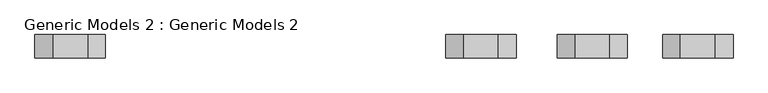
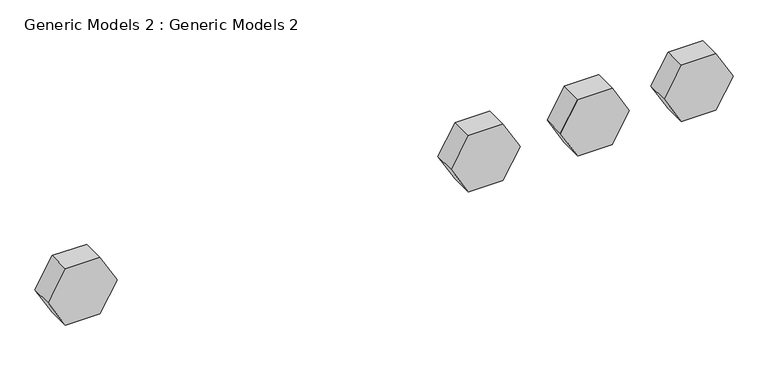
"""IFC4 building model written with IfcOpenShell, lengths in millimetres: proxy geometry, Generic Models 2 : Generic Models 2."""

from ifc_helpers import new_model, si_unit, frame, origin, place, context, project, spatial, polyline, outline, extrude, source, transform, mapped, element, save


def generic_models_2_generic_models_2_a86c904f(model_context):
    return source(origin(), model_context, "Body", "SweptSolid", [
        extrude(outline(polyline([(1234.1468146, -4720.8449167), (1234.1468146, -5178.0449167), (838.2, -5406.6449167), (442.2531854, -5178.0449167), (442.2531854, -4720.8449167), (838.2, -4492.2449167), (1234.1468146, -4720.8449167)])), frame((0.0, -8905.741091, 0.0), z_axis=(0.0, 1.0, 0.0), x_axis=(0.0, 0.0, 1.0)), (0.0, 0.0, 1.0), 304.8),
        extrude(outline(polyline([(1234.1468146, 613.1550833), (1234.1468146, 155.9550833), (838.2, -72.6449167), (442.2531854, 155.9550833), (442.2531854, 613.1550833), (838.2, 841.7550833), (1234.1468146, 613.1550833)])), frame((0.0, -8905.741091, 0.0), z_axis=(0.0, 1.0, 0.0), x_axis=(0.0, 0.0, 1.0)), (0.0, 0.0, 1.0), 304.8),
        extrude(outline(polyline([(1234.1468146, 2060.9550833), (1234.1468146, 1603.7550833), (838.2, 1375.1550833), (442.2531854, 1603.7550833), (442.2531854, 2060.9550833), (838.2, 2289.5550833), (1234.1468146, 2060.9550833)])), frame((0.0, -8905.741091, 0.0), z_axis=(0.0, 1.0, 0.0), x_axis=(0.0, 0.0, 1.0)), (0.0, 0.0, 1.0), 304.8),
        extrude(outline(polyline([(1234.1468146, 3432.5550833), (1234.1468146, 2975.3550833), (838.2, 2746.7550833), (442.2531854, 2975.3550833), (442.2531854, 3432.5550833), (838.2, 3661.1550833), (1234.1468146, 3432.5550833)])), frame((0.0, -8905.741091, 0.0), z_axis=(0.0, 1.0, 0.0), x_axis=(0.0, 0.0, 1.0)), (0.0, 0.0, 1.0), 304.8),
    ])


if __name__ == "__main__":
    model = new_model("IFC4")
    model_context = context("Model", 3, world=origin())
    ifc_project = project(units=[si_unit("LENGTHUNIT", "METRE", prefix="MILLI")], contexts=[model_context])
    site = spatial("IfcSite", under=ifc_project)
    building = spatial("IfcBuilding", under=site)
    placement = place(None, origin())
    generic_models_2_generic_models_2_shape = generic_models_2_generic_models_2_a86c904f(model_context)
    element("IfcBuildingElementProxy", 1, Name="Generic Models 2 : Generic Models 2", ObjectType="Generic Models 2 : Generic Models 2", at=placement, inside=building, context=model_context, shape_type="MappedRepresentation", body=[
        mapped(generic_models_2_generic_models_2_shape, transform((0.0, 0.0, 0.0), x_axis=(1.0, 0.0, 0.0), y_axis=(0.0, 1.0, 0.0), z_axis=(0.0, 0.0, 1.0))),
    ])
    save(model, "model.ifc")

# Revit data of these elements
# Element 1 (IfcBuildingElementProxy, "Generic Models 2 : Generic Models 2")
#   Materials on its faces: "Carpet (1)"
# Materials
#   "Carpet (1)": class "Carpet", colour RGB 124 80 67, transparency 0, Description = "Interior finish", Cost = 0
